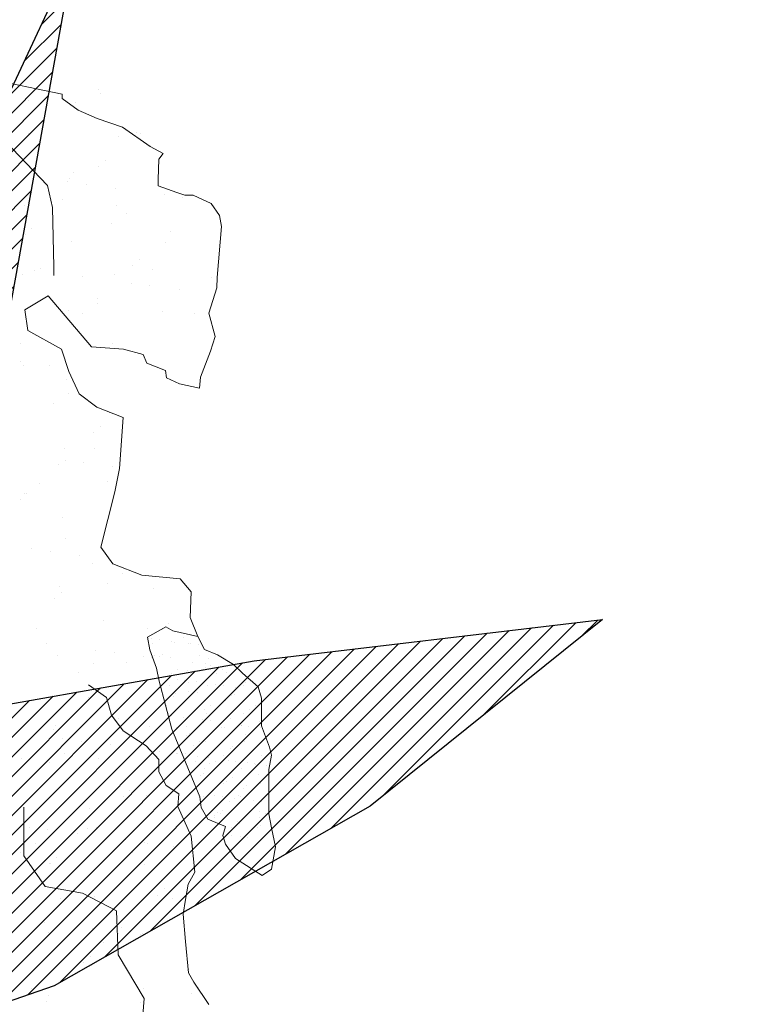
# Model space of a CAD drawing. Units: inches. Extents: x 1986 to 21484, y -1816 to 2016.
# Tile 34 of 85: x 2182.74 to 2190.96, y 1887.36 to 1898.33. Entities that reach past the tile are written whole.
import ezdxf

# ---------------------------------------------------------------- set-up
doc = ezdxf.new("R2010")
doc.units = ezdxf.units.IN
doc.layers.add('L-PLNT', color=84, linetype='Continuous', lineweight=13)
doc.layers.add('vfolhas', color=114, linetype='Continuous', lineweight=5)
doc.layers.add('vfolha2', color=110, linetype='Continuous')
doc.layers.add('vfolhas2', color=102, linetype='Continuous')
pattern_1 = [(45, (-2446.5133113, 50.986076), (-0.004419417382, 0.004419417382), [])]

# ---------------------------------------------------------------- blocks, each defined once
blk = doc.blocks.new('arbusto_PB_verde_grande')
at = {"layer": 'vfolha2'}
h = blk.add_hatch(dxfattribs=at)
h.set_pattern_fill('ANSI31', color=256, scale=0.05, style=0)
h.set_pattern_definition(pattern_1)
h.paths.add_polyline_path([(0.02944, 0.35651), (0.00028, 0.09048), (0.02625, -0.03934), (0.047, 0.06233), (0.06189, 0.09731), (0.09372, 0.26573), (0.09955, 0.43473), (0.08789, 0.61313), (0.0645, 0.72266), (0.04988, 0.6851), (0.0236, 0.51294)])
h.paths.add_polyline_path([(0.30106, 0.43789), (0.14225, 0.24871), (0.26685, 0.30022)])
h.paths.add_polyline_path([(0.37995, 0.22817), (0.23697, 0.15193), (0.18428, 0.09364), (0.11122, 0.04358), (0.02625, -0.03934), (0.28061, 0.04667), (0.36829, 0.07798), (0.46756, 0.11239), (0.61068, 0.19376), (0.71585, 0.27823), (0.55813, 0.25948)])
h.paths.add_polyline_path([(0.56101, -0.29441), (0.72752, -0.32573), (0.59024, -0.2412), (0.42962, -0.15982), (0.02625, -0.03934), (0.14922, -0.14107), (0.18838, -0.16604), (0.41501, -0.24435)])
h.paths.add_polyline_path([(-0.27429, -0.44776), (-0.30352, -0.72628), (-0.23923, -0.64175), (-0.15457, -0.45716), (0.02625, -0.03934), (-0.16328, -0.25376)])
h.paths.add_polyline_path([(-0.51963, -0.24744), (-0.67736, -0.32573), (-0.59558, -0.35072), (-0.40574, -0.32882), (-0.21007, -0.20995), (0.02625, -0.03934), (-0.14874, -0.06595), (-0.31518, -0.09101), (-0.41452, -0.15048)])
h.paths.add_polyline_path([(-0.52546, 0.25007), (-0.70947, 0.24698), (-0.51963, 0.1093), (-0.32979, 0.02167), (-0.07567, -0.0128), (-0.04234, -0.02148), (-0.35024, 0.1312)])
at = {"layer": 'vfolhas'}
h = blk.add_hatch(dxfattribs=at)
h.set_pattern_fill('ANSI31', color=256, scale=0.05, style=0)
h.set_pattern_definition(pattern_1)
h.paths.add_polyline_path([(-0.07279, 0.50669), (-0.18085, 0.65063), (-0.2334, 0.67253), (-0.20712, 0.53176), (-0.10785, 0.25007), (0.02625, -0.03934), (0.00028, 0.09048), (0.00816, 0.16241), (-0.04939, 0.29079)])
h.paths.add_polyline_path([(0.09902, 0.41929), (0.09372, 0.26573), (0.07906, 0.18814), (0.15506, 0.36901), (0.26606, 0.5505), (0.28356, 0.63504), (0.2485, 0.68819), (0.25145, 0.63504), (0.20178, 0.54426)])
h.paths.add_polyline_path([(0.12295, 0.24073), (0.047, 0.06233), (0.02625, -0.03934), (0.11122, 0.04358), (0.18428, 0.09364), (0.27478, 0.19376), (0.3215, 0.25323), (0.44129, 0.38467), (0.47634, 0.57866), (0.41789, 0.45347), (0.28939, 0.30954)])
h.paths.add_polyline_path([(0.58145, -0.03779), (0.70707, 0.01536), (0.78591, 0.04667), (0.74796, 0.06549), (0.62818, 0.08423), (0.52595, 0.09048), (0.39745, 0.04358), (0.02625, -0.03934), (0.25728, -0.03154), (0.43834, -0.0347)])
h.paths.add_polyline_path([(0.52022, -0.03647), (0.43834, -0.0347), (0.25728, -0.03154), (0.02625, -0.03934), (0.17964, -0.08515), (0.53768, -0.13167), (0.69541, -0.15357), (0.78591, -0.07852), (0.70413, -0.10042)])
h.paths.add_polyline_path([(0.27189, -0.21929), (0.14922, -0.14107), (0.02625, -0.03934), (0.15794, -0.31007), (0.29522, -0.42585), (0.41789, -0.49157), (0.56396, -0.56669), (0.5114, -0.48532), (0.39456, -0.34139)])
h.paths.add_polyline_path([(-0.05818, -0.47591), (-0.02312, -0.61984), (0.047, -0.80134), (0.08494, -0.59794), (0.07911, -0.4071), (0.03527, -0.25376), (0.02625, -0.03934), (-0.03773, -0.26001)])
h.paths.add_polyline_path([(-0.24218, 0.14054), (-0.11073, 0.06858), (0.02625, -0.03934), (-0.04235, 0.10871), (-0.21007, 0.23757), (-0.36485, 0.33145), (-0.47874, 0.40341), (-0.54303, 0.46288), (-0.49041, 0.33145), (-0.39408, 0.22192)])
at = {"layer": 'vfolha2'}
for p, q in [((0.55813, 0.25948), (0.71585, 0.27823)), ((0.71585, 0.27823), (0.61068, 0.19376)), ((0.37995, 0.22817), (0.55813, 0.25948)), ((0.61068, 0.19376), (0.46756, 0.11239))]:
    blk.add_line(p, q, dxfattribs=at)
at = {"layer": 'vfolhas2'}
for p, q in [((0.41789, 0.45347), (0.47634, 0.57866)), ((0.47634, 0.57866), (0.44129, 0.38467)), ((0.46756, 0.11239), (0.36829, 0.07798))]:
    blk.add_line(p, q, dxfattribs=at)
blk = doc.blocks.new('PLANT-SHRUB')
for p, q in [((2182.647, 1897.62), (2183.217, 1897.503)), ((2183.217, 1897.503), (2183.217, 1897.453)), ((2183.619, 1897.558), (2183.619, 1897.558)), ((2183.648, 1897.511), (2183.648, 1897.511)), ((2182.844, 1897.428), (2182.844, 1897.428)), ((2183.217, 1897.453), (2183.395, 1897.325)), ((2183.367, 1897.404), (2183.367, 1897.404)), ((2183.395, 1897.325), (2183.606, 1897.229)), ((2183.012, 1897.171), (2183.012, 1897.171)), ((2183.606, 1897.229), (2183.89, 1897.133)), ((2183.89, 1897.133), (2184.197, 1896.918)), ((2183.054, 1896.483), (2182.48, 1897.085)), ((2182.827, 1897.03), (2182.827, 1897.03)), ((2182.844, 1897.064), (2182.844, 1897.064)), ((2183.849, 1897.035), (2183.849, 1897.035)), ((2184.045, 1897.077), (2184.045, 1897.077)), ((2184.088, 1897.062), (2184.088, 1897.062)), ((2184.197, 1896.918), (2184.343, 1896.84)), ((2184.343, 1896.84), (2184.293, 1896.776)), ((2183.624, 1896.691), (2183.624, 1896.691)), ((2183.697, 1896.759), (2183.697, 1896.759)), ((2184.293, 1896.776), (2184.288, 1896.552)), ((2183.342, 1896.634), (2183.342, 1896.634)), ((2183.111, 1896.239), (2183.054, 1896.483)), ((2183.279, 1896.525), (2183.279, 1896.525)), ((2183.296, 1896.557), (2183.296, 1896.557)), ((2183.487, 1896.498), (2183.487, 1896.498)), ((2184.288, 1896.552), (2184.288, 1896.479)), ((2184.288, 1896.479), (2184.495, 1896.407)), ((2183.812, 1896.455), (2183.812, 1896.455)), ((2184.355, 1896.383), (2184.355, 1896.383)), ((2184.495, 1896.407), (2184.582, 1896.375)), ((2184.582, 1896.375), (2184.678, 1896.375)), ((2184.678, 1896.375), (2184.875, 1896.284)), ((2182.802, 1896.26), (2182.802, 1896.26)), ((2183.226, 1896.327), (2183.226, 1896.327)), ((2183.824, 1896.264), (2183.824, 1896.264)), ((2184.563, 1896.356), (2184.563, 1896.356)), ((2184.875, 1896.284), (2184.971, 1896.151)), ((2183.126, 1895.58), (2183.111, 1896.239)), ((2183.934, 1896.168), (2183.934, 1896.168)), ((2184.971, 1896.151), (2184.99, 1896.028)), ((2183.766, 1896.061), (2183.766, 1896.061)), ((2182.805, 1895.941), (2182.805, 1895.941)), ((2182.878, 1896.008), (2182.878, 1896.008)), ((2184.427, 1895.976), (2184.427, 1895.976)), ((2184.99, 1896.028), (2184.944, 1895.46)), ((2183.317, 1895.864), (2183.317, 1895.864)), ((2184.363, 1895.851), (2184.363, 1895.851)), ((2184.08, 1895.657), (2184.08, 1895.657)), ((2182.777, 1895.489), (2182.777, 1895.489)), ((2182.911, 1895.539), (2182.911, 1895.539)), ((2182.974, 1895.556), (2182.974, 1895.556)), ((2183.119, 1895.511), (2183.119, 1895.511)), ((2183.126, 1895.48), (2183.126, 1895.58)), ((2183.799, 1895.494), (2183.799, 1895.494)), ((2184.006, 1895.59), (2184.006, 1895.59)), ((2184.218, 1895.554), (2184.218, 1895.554)), ((2183.444, 1895.468), (2183.444, 1895.468)), ((2183.986, 1895.397), (2183.986, 1895.397)), ((2184.878, 1895.455), (2184.878, 1895.455)), ((2184.944, 1895.46), (2184.939, 1895.346)), ((2184.194, 1895.37), (2184.194, 1895.37)), ((2184.519, 1895.327), (2184.519, 1895.327)), ((2184.939, 1895.346), (2184.852, 1895.062)), ((2183.063, 1895.254), (2182.803, 1895.098)), ((2183.063, 1895.254), (2183.063, 1895.254)), ((2183.543, 1894.689), (2183.063, 1895.254)), ((2183.608, 1895.225), (2183.608, 1895.225)), ((2183.611, 1895.167), (2183.611, 1895.167)), ((2182.803, 1895.098), (2182.834, 1894.869)), ((2183.292, 1895.094), (2183.292, 1895.094)), ((2183.443, 1895.06), (2183.443, 1895.06)), ((2184.338, 1895.081), (2184.338, 1895.081)), ((2184.687, 1895.058), (2184.687, 1895.058)), ((2184.852, 1895.062), (2184.921, 1894.804)), ((2182.834, 1894.869), (2183.209, 1894.661)), ((2182.751, 1894.719), (2182.751, 1894.719)), ((2183.774, 1894.724), (2183.774, 1894.724)), ((2184.921, 1894.804), (2184.871, 1894.639)), ((2183.209, 1894.661), (2183.292, 1894.412)), ((2183.543, 1894.689), (2183.543, 1894.689)), ((2183.9, 1894.662), (2183.543, 1894.689)), ((2184.12, 1894.602), (2183.9, 1894.662)), ((2184.871, 1894.639), (2184.757, 1894.351)), ((2182.75, 1894.525), (2182.75, 1894.525)), ((2184.161, 1894.506), (2184.12, 1894.602)), ((2184.367, 1894.424), (2184.161, 1894.506)), ((2182.789, 1894.475), (2182.789, 1894.475)), ((2183.075, 1894.482), (2183.075, 1894.482)), ((2183.292, 1894.412), (2183.406, 1894.162)), ((2184.381, 1894.342), (2184.367, 1894.424)), ((2183.267, 1894.324), (2183.267, 1894.324)), ((2184.523, 1894.277), (2184.381, 1894.342)), ((2184.747, 1894.227), (2184.523, 1894.277)), ((2184.757, 1894.351), (2184.747, 1894.227)), ((2184.747, 1894.227), (2184.747, 1894.227)), ((2183.12, 1894.059), (2183.12, 1894.059)), ((2183.289, 1894.167), (2183.289, 1894.167)), ((2183.406, 1894.162), (2183.604, 1894.017)), ((2183.604, 1894.017), (2183.895, 1893.902)), ((2183.749, 1893.954), (2183.749, 1893.954)), ((2183.895, 1893.902), (2183.854, 1893.331)), ((2183.569, 1893.738), (2183.569, 1893.738)), ((2183.643, 1893.805), (2183.643, 1893.805)), ((2183.241, 1893.554), (2183.241, 1893.554)), ((2183.573, 1893.552), (2183.573, 1893.552)), ((2183.249, 1893.424), (2183.249, 1893.424)), ((2183.171, 1893.373), (2183.171, 1893.373)), ((2183.457, 1893.397), (2183.457, 1893.397)), ((2183.782, 1893.354), (2183.782, 1893.354)), ((2183.854, 1893.331), (2183.802, 1893.071)), ((2183.723, 1893.184), (2183.723, 1893.184)), ((2182.966, 1893.166), (2182.966, 1893.166)), ((2183.802, 1893.071), (2183.646, 1892.457)), ((2182.75, 1892.987), (2182.75, 1892.987)), ((2182.797, 1893.058), (2182.797, 1893.058)), ((2182.824, 1893.055), (2182.824, 1893.055)), ((2183.216, 1892.784), (2183.216, 1892.784)), ((2183.25, 1892.551), (2183.25, 1892.551)), ((2182.881, 1892.438), (2182.881, 1892.438)), ((2183.646, 1892.457), (2183.781, 1892.27)), ((2183.089, 1892.411), (2183.089, 1892.411)), ((2183.414, 1892.368), (2183.414, 1892.368)), ((2183.554, 1892.272), (2183.554, 1892.272)), ((2183.781, 1892.27), (2184.104, 1892.145)), ((2183.781, 1892.27), (2183.781, 1892.27)), ((2183.888, 1892.163), (2183.888, 1892.163)), ((2184.104, 1892.145), (2184.53, 1892.104)), ((2184.53, 1892.104), (2184.655, 1891.958)), ((2183.191, 1892.014), (2183.191, 1892.014)), ((2183.719, 1892.055), (2183.719, 1892.055)), ((2184.237, 1892), (2184.237, 1892)), ((2183.132, 1891.886), (2183.132, 1891.886)), ((2183.206, 1891.953), (2183.206, 1891.953)), ((2184.655, 1891.958), (2184.642, 1891.674)), ((2184.642, 1891.674), (2184.73, 1891.462)), ((2182.927, 1891.551), (2182.927, 1891.551)), ((2183.673, 1891.644), (2183.673, 1891.644)), ((2184.166, 1891.453), (2184.371, 1891.57)), ((2184.172, 1891.548), (2184.172, 1891.548)), ((2184.371, 1891.57), (2184.451, 1891.526)), ((2184.407, 1891.602), (2184.407, 1891.602)), ((2184.195, 1891.314), (2184.166, 1891.453)), ((2184.217, 1891.434), (2184.217, 1891.434)), ((2184.334, 1891.535), (2184.334, 1891.535)), ((2184.435, 1891.533), (2184.435, 1891.533)), ((2184.451, 1891.526), (2184.73, 1891.462)), ((2184.567, 1891.453), (2184.567, 1891.453)), ((2184.73, 1891.462), (2184.803, 1891.316)), ((2183.045, 1891.382), (2183.045, 1891.382)), ((2184.219, 1891.383), (2184.219, 1891.383)), ((2184.3, 1891.423), (2184.3, 1891.423)), ((2184.43, 1891.406), (2184.43, 1891.406)), ((2184.47, 1891.389), (2184.47, 1891.389)), ((2184.628, 1891.385), (2184.628, 1891.385)), ((2184.647, 1891.378), (2184.647, 1891.378)), ((2184.731, 1891.367), (2184.731, 1891.367)), ((2184.803, 1891.316), (2184.949, 1891.258)), ((2183.166, 1891.244), (2183.166, 1891.244)), ((2183.588, 1891.31), (2183.588, 1891.31)), ((2183.796, 1891.283), (2183.796, 1891.283)), ((2184.121, 1891.24), (2184.121, 1891.24)), ((2184.268, 1891.11), (2184.195, 1891.314)), ((2184.212, 1891.23), (2184.212, 1891.23)), ((2184.25, 1891.252), (2184.25, 1891.252)), ((2184.301, 1891.235), (2184.301, 1891.235)), ((2184.33, 1891.262), (2184.33, 1891.262)), ((2184.425, 1891.225), (2184.425, 1891.225)), ((2184.748, 1891.251), (2184.748, 1891.251)), ((2184.844, 1891.219), (2184.844, 1891.219)), ((2184.949, 1891.258), (2185.124, 1891.148)), ((2183.565, 1891.162), (2183.565, 1891.162)), ((2183.936, 1891.17), (2183.936, 1891.17)), ((2184.298, 1890.964), (2184.268, 1891.11)), ((2184.664, 1891.169), (2184.664, 1891.169)), ((2184.81, 1891.16), (2184.81, 1891.16)), ((2184.811, 1891.121), (2184.811, 1891.121)), ((2184.872, 1891.141), (2184.872, 1891.141)), ((2185.124, 1891.148), (2185.227, 1891.053)), ((2183.396, 1891.055), (2183.396, 1891.055)), ((2184.438, 1891.053), (2184.438, 1891.053)), ((2184.506, 1891.096), (2184.506, 1891.096)), ((2184.618, 1891.077), (2184.618, 1891.077)), ((2184.641, 1891.052), (2184.641, 1891.052)), ((2184.782, 1891.094), (2184.782, 1891.094)), ((2184.936, 1891.052), (2184.936, 1891.052)), ((2185.003, 1891.095), (2185.003, 1891.095)), ((2185.05, 1891.061), (2185.05, 1891.061)), ((2185.227, 1891.053), (2185.402, 1890.9)), ((2183.511, 1890.923), (2183.71, 1890.783)), ((2184.437, 1890.428), (2184.298, 1890.964)), ((2184.415, 1890.917), (2184.415, 1890.917)), ((2184.5, 1890.983), (2184.5, 1890.983)), ((2184.583, 1890.972), (2184.583, 1890.972)), ((2184.622, 1890.948), (2184.622, 1890.948)), ((2184.713, 1890.955), (2184.713, 1890.955)), ((2184.834, 1890.911), (2184.834, 1890.911)), ((2184.93, 1890.927), (2184.93, 1890.927)), ((2185.014, 1890.916), (2185.014, 1890.916)), ((2185.144, 1890.898), (2185.144, 1890.898)), ((2185.242, 1890.913), (2185.242, 1890.913)), ((2185.262, 1890.954), (2185.262, 1890.954)), ((2185.402, 1890.9), (2185.439, 1890.775)), ((2183.515, 1890.784), (2183.515, 1890.784)), ((2183.588, 1890.852), (2183.588, 1890.852)), ((2183.648, 1890.874), (2183.648, 1890.874)), ((2183.71, 1890.783), (2183.768, 1890.584)), ((2184.454, 1890.794), (2184.454, 1890.794)), ((2184.483, 1890.821), (2184.483, 1890.821)), ((2184.608, 1890.769), (2184.608, 1890.769)), ((2184.619, 1890.85), (2184.619, 1890.85)), ((2184.727, 1890.835), (2184.727, 1890.835)), ((2185.103, 1890.808), (2185.103, 1890.808)), ((2185.117, 1890.849), (2185.117, 1890.849)), ((2185.137, 1890.82), (2185.137, 1890.82)), ((2185.361, 1890.87), (2185.361, 1890.87)), ((2185.439, 1890.775), (2185.439, 1890.468)), ((2184.376, 1890.696), (2184.376, 1890.696)), ((2184.874, 1890.695), (2184.874, 1890.695)), ((2184.964, 1890.681), (2184.964, 1890.681)), ((2185.04, 1890.753), (2185.04, 1890.753)), ((2185.372, 1890.694), (2185.372, 1890.694)), ((2183.768, 1890.584), (2183.897, 1890.409)), ((2184.405, 1890.609), (2184.405, 1890.609)), ((2184.436, 1890.578), (2184.436, 1890.578)), ((2184.566, 1890.561), (2184.566, 1890.561)), ((2184.807, 1890.652), (2184.807, 1890.652)), ((2184.823, 1890.603), (2184.823, 1890.603)), ((2184.934, 1890.654), (2184.934, 1890.654)), ((2185.232, 1890.605), (2185.232, 1890.605)), ((2185.305, 1890.651), (2185.305, 1890.651)), ((2183.141, 1890.474), (2183.141, 1890.474)), ((2183.849, 1890.548), (2183.849, 1890.548)), ((2184.187, 1890.46), (2184.187, 1890.46)), ((2184.49, 1890.45), (2184.49, 1890.45)), ((2184.598, 1890.461), (2184.598, 1890.461)), ((2184.775, 1890.508), (2184.775, 1890.508)), ((2184.783, 1890.532), (2184.783, 1890.532)), ((2184.79, 1890.501), (2184.79, 1890.501)), ((2184.866, 1890.521), (2184.866, 1890.521)), ((2184.988, 1890.449), (2184.988, 1890.449)), ((2184.996, 1890.504), (2184.996, 1890.504)), ((2185.03, 1890.445), (2185.03, 1890.445)), ((2185.093, 1890.545), (2185.093, 1890.545)), ((2185.209, 1890.465), (2185.209, 1890.465)), ((2185.213, 1890.475), (2185.213, 1890.475)), ((2185.297, 1890.464), (2185.297, 1890.464)), ((2185.415, 1890.513), (2185.415, 1890.513)), ((2185.426, 1890.447), (2185.426, 1890.447)), ((2185.439, 1890.468), (2185.527, 1890.227)), ((2185.448, 1890.44), (2185.448, 1890.44)), ((2183.117, 1890.42), (2183.117, 1890.42)), ((2183.897, 1890.409), (2184.154, 1890.245)), ((2184.752, 1889.675), (2184.437, 1890.428)), ((2184.607, 1890.353), (2184.607, 1890.353)), ((2184.636, 1890.38), (2184.636, 1890.38)), ((2184.716, 1890.433), (2184.716, 1890.433)), ((2185.256, 1890.368), (2185.256, 1890.368)), ((2183.22, 1890.324), (2183.22, 1890.324)), ((2183.428, 1890.297), (2183.428, 1890.297)), ((2183.753, 1890.254), (2183.753, 1890.254)), ((2184.154, 1890.245), (2184.294, 1890.093)), ((2184.678, 1890.252), (2184.678, 1890.252)), ((2184.745, 1890.295), (2184.745, 1890.295)), ((2184.813, 1890.295), (2184.813, 1890.295)), ((2185.117, 1890.24), (2185.117, 1890.24)), ((2185.176, 1890.251), (2185.176, 1890.251)), ((2185.222, 1890.297), (2185.222, 1890.297)), ((2185.243, 1890.294), (2185.243, 1890.294)), ((2185.527, 1890.227), (2185.549, 1890.14)), ((2183.242, 1890.161), (2183.242, 1890.161)), ((2184.296, 1890.182), (2184.296, 1890.182)), ((2184.487, 1890.159), (2184.487, 1890.159)), ((2184.504, 1890.155), (2184.504, 1890.155)), ((2184.588, 1890.153), (2184.588, 1890.153)), ((2184.636, 1890.138), (2184.636, 1890.138)), ((2184.719, 1890.127), (2184.719, 1890.127)), ((2184.829, 1890.112), (2184.829, 1890.112)), ((2185.019, 1890.137), (2185.019, 1890.137)), ((2185.087, 1890.213), (2185.087, 1890.213)), ((2185.438, 1890.132), (2185.438, 1890.132)), ((2185.549, 1890.14), (2185.519, 1889.979)), ((2182.769, 1890.101), (2182.769, 1890.101)), ((2183.074, 1890.054), (2183.074, 1890.054)), ((2183.623, 1890.104), (2183.623, 1890.104)), ((2184.294, 1890.093), (2184.294, 1889.953)), ((2184.318, 1890.069), (2184.318, 1890.069)), ((2184.318, 1890.051), (2184.318, 1890.051)), ((2184.702, 1890.065), (2184.702, 1890.065)), ((2184.849, 1890.109), (2184.849, 1890.109)), ((2184.859, 1890.049), (2184.859, 1890.049)), ((2184.928, 1890.067), (2184.928, 1890.067)), ((2185.066, 1890.081), (2185.066, 1890.081)), ((2185.149, 1890.07), (2185.149, 1890.07)), ((2185.279, 1890.053), (2185.279, 1890.053)), ((2185.357, 1890.048), (2185.357, 1890.048)), ((2185.371, 1890.041), (2185.371, 1890.041)), ((2185.496, 1890.024), (2185.496, 1890.024)), ((2184.294, 1889.953), (2184.376, 1889.801)), ((2184.76, 1889.913), (2184.76, 1889.913)), ((2184.789, 1889.94), (2184.789, 1889.94)), ((2184.803, 1889.987), (2184.803, 1889.987)), ((2185.114, 1889.893), (2185.114, 1889.893)), ((2185.212, 1889.989), (2185.212, 1889.989)), ((2185.409, 1889.927), (2185.409, 1889.927)), ((2185.519, 1889.979), (2185.52, 1889.485)), ((2184.376, 1889.801), (2184.517, 1889.708)), ((2185.009, 1889.829), (2185.009, 1889.829)), ((2185.046, 1889.85), (2185.046, 1889.85)), ((2185.27, 1889.8), (2185.27, 1889.8)), ((2185.428, 1889.824), (2185.428, 1889.824)), ((2183.116, 1889.703), (2183.116, 1889.703)), ((2183.897, 1889.683), (2183.897, 1889.683)), ((2183.97, 1889.75), (2183.97, 1889.75)), ((2184.162, 1889.69), (2184.162, 1889.69)), ((2184.517, 1889.708), (2184.505, 1889.567)), ((2184.766, 1889.558), (2184.752, 1889.675)), ((2184.793, 1889.679), (2184.793, 1889.679)), ((2184.919, 1889.686), (2184.919, 1889.686)), ((2185.002, 1889.675), (2185.002, 1889.675)), ((2185.184, 1889.695), (2185.184, 1889.695)), ((2185.202, 1889.681), (2185.202, 1889.681)), ((2185.24, 1889.773), (2185.24, 1889.773)), ((2184.505, 1889.567), (2184.655, 1889.238)), ((2184.505, 1889.567), (2184.505, 1889.567)), ((2185.081, 1889.627), (2185.081, 1889.627)), ((2185.132, 1889.658), (2185.132, 1889.658)), ((2185.227, 1889.648), (2185.227, 1889.648)), ((2185.349, 1889.63), (2185.349, 1889.63)), ((2185.432, 1889.619), (2185.432, 1889.619)), ((2182.792, 1889.56), (2182.792, 1889.018)), ((2183.526, 1889.547), (2183.526, 1889.547)), ((2184.839, 1889.427), (2184.766, 1889.558)), ((2184.913, 1889.472), (2184.913, 1889.472)), ((2184.942, 1889.499), (2184.942, 1889.499)), ((2184.985, 1889.493), (2184.985, 1889.493)), ((2184.999, 1889.521), (2184.999, 1889.521)), ((2185.418, 1889.516), (2185.418, 1889.516)), ((2185.483, 1889.492), (2185.483, 1889.492)), ((2185.52, 1889.485), (2185.549, 1889.332)), ((2185.037, 1889.346), (2184.839, 1889.427)), ((2184.917, 1889.45), (2184.917, 1889.45)), ((2185.008, 1889.244), (2185.037, 1889.346)), ((2185.172, 1889.4), (2185.172, 1889.4)), ((2185.192, 1889.373), (2185.192, 1889.373)), ((2185.415, 1889.449), (2185.415, 1889.449)), ((2185.423, 1889.359), (2185.423, 1889.359)), ((2182.851, 1889.338), (2182.851, 1889.338)), ((2183.059, 1889.31), (2183.059, 1889.31)), ((2183.384, 1889.267), (2183.384, 1889.267)), ((2183.499, 1889.318), (2183.499, 1889.318)), ((2183.598, 1889.334), (2183.598, 1889.334)), ((2184.655, 1889.238), (2184.696, 1888.836)), ((2184.655, 1889.238), (2184.655, 1889.238)), ((2185.037, 1889.149), (2185.008, 1889.244)), ((2185.098, 1889.332), (2185.098, 1889.332)), ((2185.098, 1889.247), (2185.098, 1889.247)), ((2185.201, 1889.235), (2185.201, 1889.235)), ((2185.393, 1889.332), (2185.393, 1889.332)), ((2185.549, 1889.332), (2185.593, 1889.12)), ((2182.919, 1889.16), (2182.919, 1889.16)), ((2183.927, 1889.196), (2183.927, 1889.196)), ((2184.135, 1889.169), (2184.135, 1889.169)), ((2184.164, 1889.158), (2184.164, 1889.158)), ((2184.46, 1889.126), (2184.46, 1889.126)), ((2185.147, 1888.988), (2185.037, 1889.149)), ((2185.285, 1889.224), (2185.285, 1889.224)), ((2182.751, 1889.053), (2182.751, 1889.053)), ((2182.792, 1889.018), (2183.027, 1888.675)), ((2183.995, 1889.051), (2183.995, 1889.051)), ((2185.593, 1889.12), (2185.549, 1888.871)), ((2183.078, 1888.932), (2183.078, 1888.932)), ((2183.09, 1888.933), (2183.09, 1888.933)), ((2183.151, 1889), (2183.151, 1889)), ((2184.137, 1888.92), (2184.137, 1888.92)), ((2185.446, 1888.798), (2185.147, 1888.988)), ((2184.696, 1888.836), (2184.622, 1888.704)), ((2185.549, 1888.871), (2185.446, 1888.798)), ((2185.446, 1888.798), (2185.446, 1888.798)), ((2184.622, 1888.704), (2184.589, 1888.532)), ((2183.027, 1888.675), (2183.443, 1888.603)), ((2183.443, 1888.603), (2183.822, 1888.404)), ((2183.443, 1888.603), (2183.443, 1888.603)), ((2184.279, 1888.581), (2184.279, 1888.581)), ((2184.353, 1888.649), (2184.353, 1888.649)), ((2183.203, 1888.546), (2183.203, 1888.546)), ((2183.572, 1888.563), (2183.572, 1888.563)), ((2184.448, 1888.544), (2184.448, 1888.544)), ((2184.589, 1888.532), (2184.564, 1888.368)), ((2183.822, 1888.404), (2183.84, 1887.917)), ((2184.564, 1888.368), (2184.589, 1888.064)), ((2183.016, 1888.281), (2183.016, 1888.281)), ((2183.065, 1888.163), (2183.065, 1888.163)), ((2183.559, 1888.21), (2183.559, 1888.21)), ((2183.767, 1888.182), (2183.767, 1888.182)), ((2183.841, 1888.157), (2183.841, 1888.157)), ((2183.881, 1888.217), (2183.881, 1888.217)), ((2184.092, 1888.14), (2184.092, 1888.14)), ((2184.111, 1888.15), (2184.111, 1888.15)), ((2183.673, 1888.05), (2183.673, 1888.05)), ((2184.589, 1888.064), (2184.626, 1887.716)), ((2183.84, 1887.917), (2184.129, 1887.429)), ((2183.46, 1887.831), (2183.46, 1887.831)), ((2183.534, 1887.898), (2183.534, 1887.898)), ((2183.547, 1887.793), (2183.547, 1887.793)), ((2184.626, 1887.716), (2184.684, 1887.612)), ((2184.627, 1887.755), (2184.627, 1887.755)), ((2184.684, 1887.612), (2184.851, 1887.364)), ((2182.88, 1887.545), (2182.88, 1887.545)), ((2184.125, 1887.543), (2184.125, 1887.543)), ((2184.661, 1887.48), (2184.661, 1887.48)), ((2184.735, 1887.547), (2184.735, 1887.547)), ((2183.04, 1887.393), (2183.04, 1887.393)), ((2183.062, 1887.466), (2183.062, 1887.466)), ((2184.086, 1887.38), (2184.086, 1887.38)), ((2184.129, 1887.429), (2184.111, 1887.195))]:
    blk.add_line(p, q)

msp = doc.modelspace()

# ---------------------------------------------------------------- block references
at = {"layer": 'L-PLNT'}
msp.add_blockref('PLANT-SHRUB', (0, 0), dxfattribs=at)
at = {"layer": 'L-PLNT', "xscale": 24.60366729364114, "yscale": 24.60366729364114, "zscale": 24.60366729364114}
msp.add_blockref('arbusto_PB_verde_grande', (2171.623, 1884.805), dxfattribs=at)

doc.saveas('drawing.dxf')
